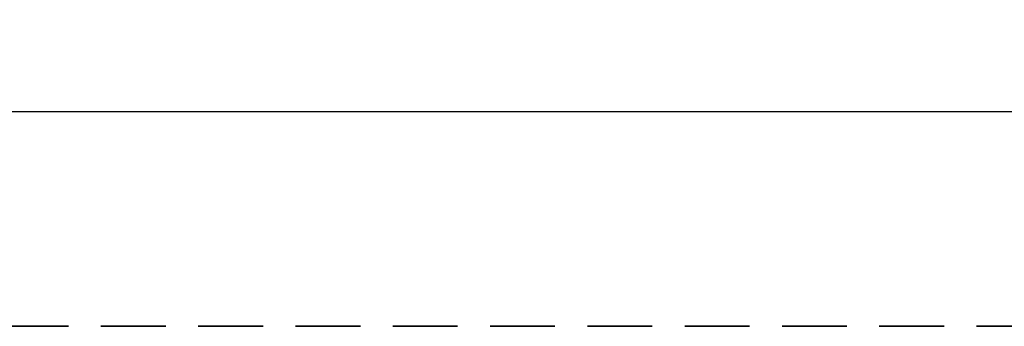
# Model space of a CAD drawing. Units: inches. Extents: x -7 to 1228, y -146 to 1091.
# Tile 56 of 88: x 96 to 193, y 1061 to 1091. Entities that reach past the tile are written whole.
import ezdxf

# ---------------------------------------------------------------- set-up
doc = ezdxf.new("R2010")
doc.units = ezdxf.units.IN
doc.linetypes.add('DASHED2', pattern=[9.525, 6.35, -3.175])
doc.layers.add('A-ANNO-DIMS', color=2, linetype='Continuous', lineweight=18)
doc.layers.add('C-PROP', color=1, linetype='DASHED2', lineweight=35)
doc.styles.get("Standard").update_dxf_attribs({"font": 'arial.ttf'})
doc.dimstyles.new('ISO-25', dxfattribs={"dimtxt": 7, "dimasz": 4, "dimexe": 1.25, "dimexo": 0.625, "dimtad": 1, "dimdec": 1, "dimlunit": 3, "dimtxsty": 'Standard', "dimcen": 2.5, "dimadec": 0, "dimazin": 0, "dimtfac": 1, "dimtdec": 1, "dimtmove": 1, "dimatfit": 3, "dimfxl": 1, "dimarcsym": 0})

# ---------------------------------------------------------------- blocks, each defined once
blk = doc.blocks.new('*D11')
at = {"layer": 'A-ANNO-DIMS', "color": 0, "lineweight": -2, "transparency": 16777216}
for p, q in [((0, 1061.625), (0, 1083.25)), ((1187, 1061.625), (1187, 1083.25)), ((4, 1082), (1183, 1082))]:
    blk.add_line(p, q, dxfattribs=at)
at = {"layer": 'A-ANNO-DIMS', "color": 0, "transparency": 16777216}
for points in [[(4, 1082.667), (4, 1081.333), (0, 1082)], [(1183, 1082.667), (1183, 1081.333), (1187, 1082)]]:
    blk.add_solid(points, dxfattribs=at)
at = {"layer": 'Defpoints', "color": 0, "transparency": 16777216}
for p in [(1187, 1082), (0, 1061), (1187, 1061)]:
    blk.add_point(p, dxfattribs=at)
at = {"layer": 'A-ANNO-DIMS', "color": 0, "transparency": 16777216, "insert": (593.5, 1086.199), "char_height": 7, "attachment_point": 5}
blk.add_mtext('98\'-11"', dxfattribs=at)

msp = doc.modelspace()

# ---------------------------------------------------------------- linework, layer by layer
at = {"layer": 'C-PROP'}
msp.add_line((1187, 1061), (0, 1061), dxfattribs=at)

# ---------------------------------------------------------------- dimensions: what is measured, and where the dimension line sits
at = {"layer": 'A-ANNO-DIMS'}
dim = msp.add_linear_dim(base=(1187, 1082), p1=(0, 1061), p2=(1187, 1061), dimstyle='ISO-25', override={"dimclrd": 0, "dimclre": 0, "dimclrt": 0}, dxfattribs=at)
dim.commit()
dim.dimension.update_dxf_attribs({"geometry": '*D11', "text_midpoint": (593.5, 1086.199)})

doc.saveas('drawing.dxf')
